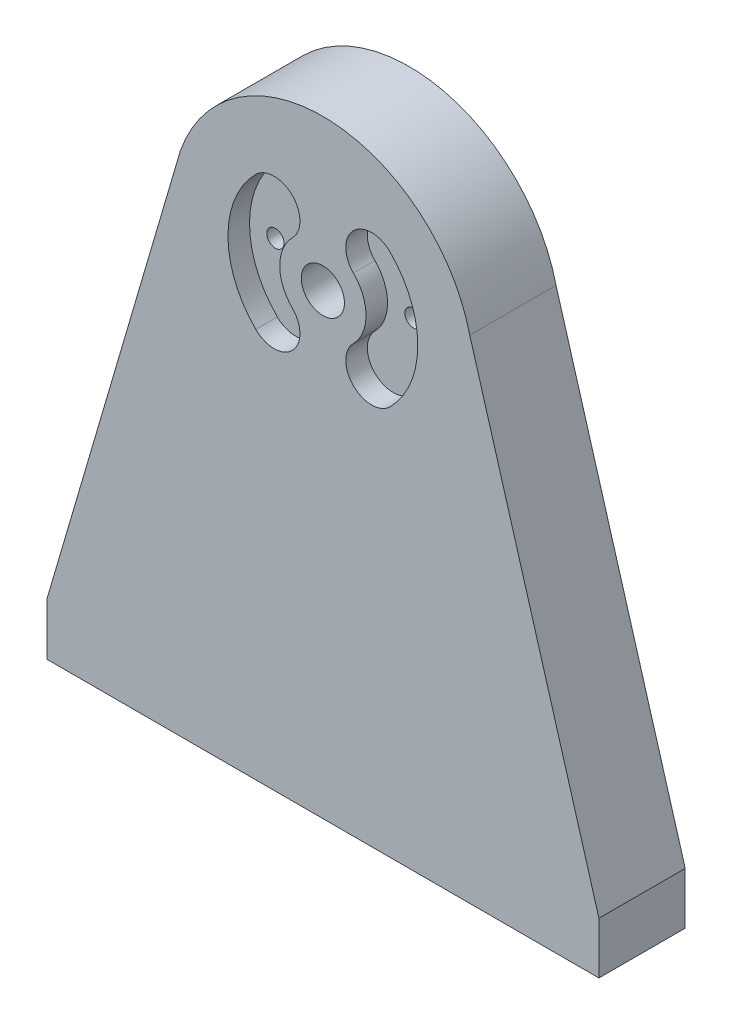
ISO-10303-21;
HEADER;
FILE_DESCRIPTION(('STEP AP214'),'2;1');
FILE_NAME('part.step','',(''),(''),'','','');
FILE_SCHEMA(('AUTOMOTIVE_DESIGN { 1 0 10303 214 1 1 1 1 }'));
ENDSEC;
DATA;
#1=APPLICATION_CONTEXT('core data for automotive mechanical design processes');
#2=APPLICATION_PROTOCOL_DEFINITION('international standard','automotive_design',2000,#1);
#3=PRODUCT_CONTEXT('',#1,'mechanical');
#4=PRODUCT('Part','Part','',(#3));
#5=PRODUCT_RELATED_PRODUCT_CATEGORY('part','',(#4));
#6=PRODUCT_DEFINITION_FORMATION('','',#4);
#7=PRODUCT_DEFINITION_CONTEXT('part definition',#1,'design');
#8=PRODUCT_DEFINITION('design','',#6,#7);
#9=PRODUCT_DEFINITION_SHAPE('','',#8);
#10=(LENGTH_UNIT() NAMED_UNIT(*) SI_UNIT(.MILLI.,.METRE.));
#11=(NAMED_UNIT(*) PLANE_ANGLE_UNIT() SI_UNIT($,.RADIAN.));
#12=(NAMED_UNIT(*) SI_UNIT($,.STERADIAN.) SOLID_ANGLE_UNIT());
#13=UNCERTAINTY_MEASURE_WITH_UNIT(LENGTH_MEASURE(1.E-05),#10,'distance_accuracy_value','');
#14=(GEOMETRIC_REPRESENTATION_CONTEXT(3) GLOBAL_UNCERTAINTY_ASSIGNED_CONTEXT((#13)) GLOBAL_UNIT_ASSIGNED_CONTEXT((#10,
#11,#12)) REPRESENTATION_CONTEXT('',''));
#15=CARTESIAN_POINT('',(0.,0.,0.));
#16=DIRECTION('',(0.,0.,1.));
#17=DIRECTION('',(1.,0.,0.));
#18=AXIS2_PLACEMENT_3D('',#15,#16,#17);
#19=CARTESIAN_POINT('',(8.,55.,5.));
#20=DIRECTION('',(0.,-1.,0.));
#21=DIRECTION('',(0.,0.,-1.));
#22=AXIS2_PLACEMENT_3D('',#19,#20,#21);
#23=CYLINDRICAL_SURFACE('',#22,1.);
#24=CARTESIAN_POINT('',(8.,0.,5.));
#25=DIRECTION('',(0.,-1.,0.));
#26=DIRECTION('',(0.,0.,-1.));
#27=AXIS2_PLACEMENT_3D('',#24,#25,#26);
#28=CIRCLE('',#27,1.);
#29=CARTESIAN_POINT('',(8.,0.,4.));
#30=VERTEX_POINT('',#29);
#31=EDGE_CURVE('E264',#30,#30,#28,.T.);
#32=ORIENTED_EDGE('',*,*,#31,.T.);
#33=EDGE_LOOP('',(#32));
#34=FACE_BOUND('',#33,.T.);
#35=CARTESIAN_POINT('',(8.,53.,5.));
#36=DIRECTION('',(0.,-0.707106781186547,-0.707106781186547));
#37=DIRECTION('',(0.,-0.707106781186547,0.707106781186547));
#38=AXIS2_PLACEMENT_3D('',#35,#36,#37);
#39=ELLIPSE('',#38,1.4142135623731,1.);
#40=CARTESIAN_POINT('',(7.,53.,5.));
#41=VERTEX_POINT('',#40);
#42=CARTESIAN_POINT('',(9.,53.,5.));
#43=VERTEX_POINT('',#42);
#44=EDGE_CURVE('E62',#41,#43,#39,.F.);
#45=ORIENTED_EDGE('',*,*,#44,.T.);
#46=CARTESIAN_POINT('',(8.,53.,5.));
#47=DIRECTION('',(0.,-0.707106781186547,0.707106781186547));
#48=DIRECTION('',(0.,-0.707106781186547,-0.707106781186547));
#49=AXIS2_PLACEMENT_3D('',#46,#47,#48);
#50=ELLIPSE('',#49,1.4142135623731,1.);
#51=EDGE_CURVE('E187',#43,#41,#50,.F.);
#52=ORIENTED_EDGE('',*,*,#51,.T.);
#53=EDGE_LOOP('',(#45,#52));
#54=FACE_BOUND('',#53,.T.);
#55=ADVANCED_FACE('F44',(#34,#54),#23,.F.);
#56=CARTESIAN_POINT('',(-8.,55.,5.));
#57=DIRECTION('',(0.,-1.,0.));
#58=DIRECTION('',(0.,0.,-1.));
#59=AXIS2_PLACEMENT_3D('',#56,#57,#58);
#60=CYLINDRICAL_SURFACE('',#59,1.);
#61=CARTESIAN_POINT('',(-8.,0.,5.));
#62=DIRECTION('',(0.,-1.,0.));
#63=DIRECTION('',(0.,0.,-1.));
#64=AXIS2_PLACEMENT_3D('',#61,#62,#63);
#65=CIRCLE('',#64,1.);
#66=CARTESIAN_POINT('',(-8.,0.,4.));
#67=VERTEX_POINT('',#66);
#68=EDGE_CURVE('E259',#67,#67,#65,.T.);
#69=ORIENTED_EDGE('',*,*,#68,.T.);
#70=EDGE_LOOP('',(#69));
#71=FACE_BOUND('',#70,.T.);
#72=CARTESIAN_POINT('',(-8.,53.,5.));
#73=DIRECTION('',(0.,-0.707106781186547,-0.707106781186547));
#74=DIRECTION('',(0.,-0.707106781186547,0.707106781186547));
#75=AXIS2_PLACEMENT_3D('',#72,#73,#74);
#76=ELLIPSE('',#75,1.41421356237309,1.);
#77=CARTESIAN_POINT('',(-9.,53.,5.));
#78=VERTEX_POINT('',#77);
#79=CARTESIAN_POINT('',(-7.,53.,5.));
#80=VERTEX_POINT('',#79);
#81=EDGE_CURVE('E69',#78,#80,#76,.F.);
#82=ORIENTED_EDGE('',*,*,#81,.T.);
#83=CARTESIAN_POINT('',(-8.,53.,5.));
#84=DIRECTION('',(0.,-0.707106781186547,0.707106781186547));
#85=DIRECTION('',(0.,-0.707106781186547,-0.707106781186547));
#86=AXIS2_PLACEMENT_3D('',#83,#84,#85);
#87=ELLIPSE('',#86,1.41421356237309,1.);
#88=EDGE_CURVE('E163',#80,#78,#87,.F.);
#89=ORIENTED_EDGE('',*,*,#88,.T.);
#90=EDGE_LOOP('',(#82,#89));
#91=FACE_BOUND('',#90,.T.);
#92=ADVANCED_FACE('F173',(#71,#91),#60,.F.);
#93=CARTESIAN_POINT('',(0.,53.,10.));
#94=DIRECTION('',(0.,0.,1.));
#95=DIRECTION('',(1.,0.,0.));
#96=AXIS2_PLACEMENT_3D('',#93,#94,#95);
#97=PLANE('',#96);
#98=CARTESIAN_POINT('',(5.65685424949238,58.6568542494924,10.));
#99=DIRECTION('',(0.,0.,1.));
#100=DIRECTION('',(-1.,0.,0.));
#101=AXIS2_PLACEMENT_3D('',#98,#99,#100);
#102=CIRCLE('',#101,3.);
#103=CARTESIAN_POINT('',(7.77817459305203,60.778174593052,10.));
#104=VERTEX_POINT('',#103);
#105=CARTESIAN_POINT('',(3.53553390593274,56.5355339059327,10.));
#106=VERTEX_POINT('',#105);
#107=EDGE_CURVE('E188',#104,#106,#102,.T.);
#108=ORIENTED_EDGE('',*,*,#107,.F.);
#109=CARTESIAN_POINT('',(0.,53.,10.));
#110=DIRECTION('',(0.,0.,1.));
#111=DIRECTION('',(1.,0.,0.));
#112=AXIS2_PLACEMENT_3D('',#109,#110,#111);
#113=CIRCLE('',#112,11.);
#114=CARTESIAN_POINT('',(7.77817459305202,45.221825406948,10.));
#115=VERTEX_POINT('',#114);
#116=EDGE_CURVE('E230',#115,#104,#113,.T.);
#117=ORIENTED_EDGE('',*,*,#116,.F.);
#118=CARTESIAN_POINT('',(5.65685424949238,47.3431457505076,10.));
#119=DIRECTION('',(0.,0.,1.));
#120=DIRECTION('',(1.,0.,0.));
#121=AXIS2_PLACEMENT_3D('',#118,#119,#120);
#122=CIRCLE('',#121,3.);
#123=CARTESIAN_POINT('',(3.53553390593273,49.4644660940673,10.));
#124=VERTEX_POINT('',#123);
#125=EDGE_CURVE('E242',#124,#115,#122,.T.);
#126=ORIENTED_EDGE('',*,*,#125,.F.);
#127=CARTESIAN_POINT('',(0.,53.,10.));
#128=DIRECTION('',(0.,0.,-1.));
#129=DIRECTION('',(1.,0.,0.));
#130=AXIS2_PLACEMENT_3D('',#127,#128,#129);
#131=CIRCLE('',#130,5.);
#132=EDGE_CURVE('E236',#106,#124,#131,.T.);
#133=ORIENTED_EDGE('',*,*,#132,.F.);
#134=EDGE_LOOP('',(#108,#117,#126,#133));
#135=FACE_BOUND('',#134,.T.);
#136=CARTESIAN_POINT('',(0.,53.,10.));
#137=DIRECTION('',(0.,0.,1.));
#138=DIRECTION('',(1.,0.,0.));
#139=AXIS2_PLACEMENT_3D('',#136,#137,#138);
#140=CIRCLE('',#139,2.5);
#141=CARTESIAN_POINT('',(2.5,53.,10.));
#142=VERTEX_POINT('',#141);
#143=EDGE_CURVE('E216',#142,#142,#140,.T.);
#144=ORIENTED_EDGE('',*,*,#143,.F.);
#145=EDGE_LOOP('',(#144));
#146=FACE_BOUND('',#145,.T.);
#147=DIRECTION('',(-0.281490106882961,0.959564130075223,0.));
#148=VECTOR('',#147,1.);
#149=CARTESIAN_POINT('',(32.,6.,10.));
#150=LINE('',#149,#148);
#151=CARTESIAN_POINT('',(32.,6.,10.));
#152=VERTEX_POINT('',#151);
#153=CARTESIAN_POINT('',(17.027168618915,57.0404862112172,10.));
#154=VERTEX_POINT('',#153);
#155=EDGE_CURVE('E289',#152,#154,#150,.T.);
#156=ORIENTED_EDGE('',*,*,#155,.T.);
#157=CARTESIAN_POINT('',(0.,53.,10.));
#158=DIRECTION('',(0.,0.,1.));
#159=DIRECTION('',(1.,0.,0.));
#160=AXIS2_PLACEMENT_3D('',#157,#158,#159);
#161=CIRCLE('',#160,17.5);
#162=CARTESIAN_POINT('',(-16.5115497472368,58.7981656534221,10.));
#163=VERTEX_POINT('',#162);
#164=EDGE_CURVE('E292',#154,#163,#161,.T.);
#165=ORIENTED_EDGE('',*,*,#164,.T.);
#166=DIRECTION('',(-0.281490106882961,-0.959564130075223,0.));
#167=VECTOR('',#166,1.);
#168=CARTESIAN_POINT('',(-32.,6.,10.));
#169=LINE('',#168,#167);
#170=CARTESIAN_POINT('',(-32.,6.,10.));
#171=VERTEX_POINT('',#170);
#172=EDGE_CURVE('E294',#163,#171,#169,.T.);
#173=ORIENTED_EDGE('',*,*,#172,.T.);
#174=DIRECTION('',(0.,-1.,0.));
#175=VECTOR('',#174,1.);
#176=CARTESIAN_POINT('',(-32.,0.,10.));
#177=LINE('',#176,#175);
#178=CARTESIAN_POINT('',(-32.,0.,10.));
#179=VERTEX_POINT('',#178);
#180=EDGE_CURVE('E297',#171,#179,#177,.T.);
#181=ORIENTED_EDGE('',*,*,#180,.T.);
#182=DIRECTION('',(1.,0.,0.));
#183=VECTOR('',#182,1.);
#184=CARTESIAN_POINT('',(-32.,0.,10.));
#185=LINE('',#184,#183);
#186=CARTESIAN_POINT('',(32.,0.,10.));
#187=VERTEX_POINT('',#186);
#188=EDGE_CURVE('E298',#179,#187,#185,.T.);
#189=ORIENTED_EDGE('',*,*,#188,.T.);
#190=DIRECTION('',(0.,1.,0.));
#191=VECTOR('',#190,1.);
#192=CARTESIAN_POINT('',(32.,0.,10.));
#193=LINE('',#192,#191);
#194=EDGE_CURVE('E296',#187,#152,#193,.T.);
#195=ORIENTED_EDGE('',*,*,#194,.T.);
#196=EDGE_LOOP('',(#156,#165,#173,#181,#189,#195));
#197=FACE_BOUND('',#196,.T.);
#198=CARTESIAN_POINT('',(-5.65685424949238,47.3431457505076,10.));
#199=DIRECTION('',(0.,0.,1.));
#200=DIRECTION('',(-1.,0.,0.));
#201=AXIS2_PLACEMENT_3D('',#198,#199,#200);
#202=CIRCLE('',#201,3.);
#203=CARTESIAN_POINT('',(-7.77817459305202,45.221825406948,10.));
#204=VERTEX_POINT('',#203);
#205=CARTESIAN_POINT('',(-3.53553390593274,49.4644660940673,10.));
#206=VERTEX_POINT('',#205);
#207=EDGE_CURVE('E201',#204,#206,#202,.T.);
#208=ORIENTED_EDGE('',*,*,#207,.F.);
#209=CARTESIAN_POINT('',(0.,53.,10.));
#210=DIRECTION('',(0.,0.,1.));
#211=DIRECTION('',(1.,0.,0.));
#212=AXIS2_PLACEMENT_3D('',#209,#210,#211);
#213=CIRCLE('',#212,11.);
#214=CARTESIAN_POINT('',(-7.77817459305202,60.778174593052,10.));
#215=VERTEX_POINT('',#214);
#216=EDGE_CURVE('E194',#215,#204,#213,.T.);
#217=ORIENTED_EDGE('',*,*,#216,.F.);
#218=CARTESIAN_POINT('',(-5.65685424949238,58.6568542494924,10.));
#219=DIRECTION('',(0.,0.,1.));
#220=DIRECTION('',(1.,0.,0.));
#221=AXIS2_PLACEMENT_3D('',#218,#219,#220);
#222=CIRCLE('',#221,3.);
#223=CARTESIAN_POINT('',(-3.53553390593274,56.5355339059327,10.));
#224=VERTEX_POINT('',#223);
#225=EDGE_CURVE('E207',#224,#215,#222,.T.);
#226=ORIENTED_EDGE('',*,*,#225,.F.);
#227=CARTESIAN_POINT('',(0.,53.,10.));
#228=DIRECTION('',(0.,0.,-1.));
#229=DIRECTION('',(1.,0.,0.));
#230=AXIS2_PLACEMENT_3D('',#227,#228,#229);
#231=CIRCLE('',#230,5.00000000000001);
#232=EDGE_CURVE('E202',#206,#224,#231,.T.);
#233=ORIENTED_EDGE('',*,*,#232,.F.);
#234=EDGE_LOOP('',(#208,#217,#226,#233));
#235=FACE_BOUND('',#234,.T.);
#236=ADVANCED_FACE('F371',(#135,#146,#197,#235),#97,.T.);
#237=CARTESIAN_POINT('',(32.,6.,10.));
#238=DIRECTION('',(-0.959564130075223,-0.281490106882961,0.));
#239=DIRECTION('',(0.281490106882961,-0.959564130075223,0.));
#240=AXIS2_PLACEMENT_3D('',#237,#238,#239);
#241=PLANE('',#240);
#242=DIRECTION('',(-0.281490106882961,0.959564130075223,0.));
#243=VECTOR('',#242,1.);
#244=CARTESIAN_POINT('',(32.,6.,0.));
#245=LINE('',#244,#243);
#246=CARTESIAN_POINT('',(32.,6.,0.));
#247=VERTEX_POINT('',#246);
#248=CARTESIAN_POINT('',(17.027168618915,57.0404862112172,0.));
#249=VERTEX_POINT('',#248);
#250=EDGE_CURVE('E280',#247,#249,#245,.T.);
#251=ORIENTED_EDGE('',*,*,#250,.T.);
#252=DIRECTION('',(0.,0.,-1.));
#253=VECTOR('',#252,1.);
#254=CARTESIAN_POINT('',(17.027168618915,57.0404862112172,10.));
#255=LINE('',#254,#253);
#256=EDGE_CURVE('E11',#154,#249,#255,.T.);
#257=ORIENTED_EDGE('',*,*,#256,.F.);
#258=ORIENTED_EDGE('',*,*,#155,.F.);
#259=DIRECTION('',(0.,0.,-1.));
#260=VECTOR('',#259,1.);
#261=CARTESIAN_POINT('',(32.,6.,10.));
#262=LINE('',#261,#260);
#263=EDGE_CURVE('E305',#152,#247,#262,.T.);
#264=ORIENTED_EDGE('',*,*,#263,.T.);
#265=EDGE_LOOP('',(#251,#257,#258,#264));
#266=FACE_BOUND('',#265,.T.);
#267=ADVANCED_FACE('F50',(#266),#241,.F.);
#268=CARTESIAN_POINT('',(0.,53.,10.));
#269=DIRECTION('',(0.,0.,-1.));
#270=DIRECTION('',(-1.,0.,0.));
#271=AXIS2_PLACEMENT_3D('',#268,#269,#270);
#272=CYLINDRICAL_SURFACE('',#271,17.5);
#273=CARTESIAN_POINT('',(0.,53.,0.));
#274=DIRECTION('',(0.,0.,1.));
#275=DIRECTION('',(1.,0.,0.));
#276=AXIS2_PLACEMENT_3D('',#273,#274,#275);
#277=CIRCLE('',#276,17.5);
#278=CARTESIAN_POINT('',(-16.5115497472368,58.7981656534221,0.));
#279=VERTEX_POINT('',#278);
#280=EDGE_CURVE('E303',#249,#279,#277,.T.);
#281=ORIENTED_EDGE('',*,*,#280,.T.);
#282=DIRECTION('',(0.,0.,-1.));
#283=VECTOR('',#282,1.);
#284=CARTESIAN_POINT('',(-16.5115497472368,58.7981656534221,10.));
#285=LINE('',#284,#283);
#286=EDGE_CURVE('E53',#163,#279,#285,.T.);
#287=ORIENTED_EDGE('',*,*,#286,.F.);
#288=ORIENTED_EDGE('',*,*,#164,.F.);
#289=ORIENTED_EDGE('',*,*,#256,.T.);
#290=EDGE_LOOP('',(#281,#287,#288,#289));
#291=FACE_BOUND('',#290,.T.);
#292=ADVANCED_FACE('F381',(#291),#272,.T.);
#293=CARTESIAN_POINT('',(-32.,6.,10.));
#294=DIRECTION('',(0.959564130075223,-0.281490106882961,0.));
#295=DIRECTION('',(0.281490106882961,0.959564130075223,0.));
#296=AXIS2_PLACEMENT_3D('',#293,#294,#295);
#297=PLANE('',#296);
#298=DIRECTION('',(-0.281490106882961,-0.959564130075223,0.));
#299=VECTOR('',#298,1.);
#300=CARTESIAN_POINT('',(-32.,6.,0.));
#301=LINE('',#300,#299);
#302=CARTESIAN_POINT('',(-32.,6.,0.));
#303=VERTEX_POINT('',#302);
#304=EDGE_CURVE('E307',#279,#303,#301,.T.);
#305=ORIENTED_EDGE('',*,*,#304,.T.);
#306=DIRECTION('',(0.,0.,-1.));
#307=VECTOR('',#306,1.);
#308=CARTESIAN_POINT('',(-32.,6.,10.));
#309=LINE('',#308,#307);
#310=EDGE_CURVE('E325',#171,#303,#309,.T.);
#311=ORIENTED_EDGE('',*,*,#310,.F.);
#312=ORIENTED_EDGE('',*,*,#172,.F.);
#313=ORIENTED_EDGE('',*,*,#286,.T.);
#314=EDGE_LOOP('',(#305,#311,#312,#313));
#315=FACE_BOUND('',#314,.T.);
#316=ADVANCED_FACE('F377',(#315),#297,.F.);
#317=CARTESIAN_POINT('',(-32.,0.,10.));
#318=DIRECTION('',(1.,0.,0.));
#319=DIRECTION('',(0.,0.,-1.));
#320=AXIS2_PLACEMENT_3D('',#317,#318,#319);
#321=PLANE('',#320);
#322=DIRECTION('',(0.,-1.,0.));
#323=VECTOR('',#322,1.);
#324=CARTESIAN_POINT('',(-32.,0.,0.));
#325=LINE('',#324,#323);
#326=CARTESIAN_POINT('',(-32.,0.,0.));
#327=VERTEX_POINT('',#326);
#328=EDGE_CURVE('E310',#303,#327,#325,.T.);
#329=ORIENTED_EDGE('',*,*,#328,.T.);
#330=DIRECTION('',(0.,0.,-1.));
#331=VECTOR('',#330,1.);
#332=CARTESIAN_POINT('',(-32.,0.,10.));
#333=LINE('',#332,#331);
#334=EDGE_CURVE('E317',#179,#327,#333,.T.);
#335=ORIENTED_EDGE('',*,*,#334,.F.);
#336=ORIENTED_EDGE('',*,*,#180,.F.);
#337=ORIENTED_EDGE('',*,*,#310,.T.);
#338=EDGE_LOOP('',(#329,#335,#336,#337));
#339=FACE_BOUND('',#338,.T.);
#340=ADVANCED_FACE('F355',(#339),#321,.F.);
#341=CARTESIAN_POINT('',(-32.,0.,10.));
#342=DIRECTION('',(0.,1.,0.));
#343=DIRECTION('',(0.,0.,1.));
#344=AXIS2_PLACEMENT_3D('',#341,#342,#343);
#345=PLANE('',#344);
#346=ORIENTED_EDGE('',*,*,#68,.F.);
#347=EDGE_LOOP('',(#346));
#348=FACE_BOUND('',#347,.T.);
#349=ORIENTED_EDGE('',*,*,#31,.F.);
#350=EDGE_LOOP('',(#349));
#351=FACE_BOUND('',#350,.T.);
#352=CARTESIAN_POINT('',(22.,0.,5.));
#353=DIRECTION('',(0.,-1.,0.));
#354=DIRECTION('',(0.,0.,-1.));
#355=AXIS2_PLACEMENT_3D('',#352,#353,#354);
#356=CIRCLE('',#355,2.5);
#357=CARTESIAN_POINT('',(22.,0.,2.5));
#358=VERTEX_POINT('',#357);
#359=EDGE_CURVE('E279',#358,#358,#356,.T.);
#360=ORIENTED_EDGE('',*,*,#359,.F.);
#361=EDGE_LOOP('',(#360));
#362=FACE_BOUND('',#361,.T.);
#363=CARTESIAN_POINT('',(-22.,0.,5.));
#364=DIRECTION('',(0.,-1.,0.));
#365=DIRECTION('',(0.,0.,-1.));
#366=AXIS2_PLACEMENT_3D('',#363,#364,#365);
#367=CIRCLE('',#366,2.5);
#368=CARTESIAN_POINT('',(-22.,0.,2.5));
#369=VERTEX_POINT('',#368);
#370=EDGE_CURVE('E284',#369,#369,#367,.T.);
#371=ORIENTED_EDGE('',*,*,#370,.F.);
#372=EDGE_LOOP('',(#371));
#373=FACE_BOUND('',#372,.T.);
#374=DIRECTION('',(1.,0.,0.));
#375=VECTOR('',#374,1.);
#376=CARTESIAN_POINT('',(-32.,0.,0.));
#377=LINE('',#376,#375);
#378=CARTESIAN_POINT('',(32.,0.,0.));
#379=VERTEX_POINT('',#378);
#380=EDGE_CURVE('E313',#327,#379,#377,.T.);
#381=ORIENTED_EDGE('',*,*,#380,.T.);
#382=DIRECTION('',(0.,0.,-1.));
#383=VECTOR('',#382,1.);
#384=CARTESIAN_POINT('',(32.,0.,10.));
#385=LINE('',#384,#383);
#386=EDGE_CURVE('E316',#187,#379,#385,.T.);
#387=ORIENTED_EDGE('',*,*,#386,.F.);
#388=ORIENTED_EDGE('',*,*,#188,.F.);
#389=ORIENTED_EDGE('',*,*,#334,.T.);
#390=EDGE_LOOP('',(#381,#387,#388,#389));
#391=FACE_BOUND('',#390,.T.);
#392=ADVANCED_FACE('F346',(#348,#351,#362,#373,#391),#345,.F.);
#393=CARTESIAN_POINT('',(32.,0.,10.));
#394=DIRECTION('',(-1.,0.,0.));
#395=DIRECTION('',(0.,0.,1.));
#396=AXIS2_PLACEMENT_3D('',#393,#394,#395);
#397=PLANE('',#396);
#398=DIRECTION('',(0.,1.,0.));
#399=VECTOR('',#398,1.);
#400=CARTESIAN_POINT('',(32.,0.,0.));
#401=LINE('',#400,#399);
#402=EDGE_CURVE('E295',#379,#247,#401,.T.);
#403=ORIENTED_EDGE('',*,*,#402,.T.);
#404=ORIENTED_EDGE('',*,*,#263,.F.);
#405=ORIENTED_EDGE('',*,*,#194,.F.);
#406=ORIENTED_EDGE('',*,*,#386,.T.);
#407=EDGE_LOOP('',(#403,#404,#405,#406));
#408=FACE_BOUND('',#407,.T.);
#409=ADVANCED_FACE('F352',(#408),#397,.F.);
#410=CARTESIAN_POINT('',(0.,53.,0.));
#411=DIRECTION('',(0.,0.,1.));
#412=DIRECTION('',(1.,0.,0.));
#413=AXIS2_PLACEMENT_3D('',#410,#411,#412);
#414=PLANE('',#413);
#415=CARTESIAN_POINT('',(0.,53.,0.));
#416=DIRECTION('',(0.,0.,1.));
#417=DIRECTION('',(1.,0.,0.));
#418=AXIS2_PLACEMENT_3D('',#415,#416,#417);
#419=CIRCLE('',#418,2.5);
#420=CARTESIAN_POINT('',(2.5,53.,0.));
#421=VERTEX_POINT('',#420);
#422=EDGE_CURVE('E47',#421,#421,#419,.T.);
#423=ORIENTED_EDGE('',*,*,#422,.T.);
#424=EDGE_LOOP('',(#423));
#425=FACE_BOUND('',#424,.T.);
#426=ORIENTED_EDGE('',*,*,#250,.F.);
#427=ORIENTED_EDGE('',*,*,#402,.F.);
#428=ORIENTED_EDGE('',*,*,#380,.F.);
#429=ORIENTED_EDGE('',*,*,#328,.F.);
#430=ORIENTED_EDGE('',*,*,#304,.F.);
#431=ORIENTED_EDGE('',*,*,#280,.F.);
#432=EDGE_LOOP('',(#426,#427,#428,#429,#430,#431));
#433=FACE_BOUND('',#432,.T.);
#434=ADVANCED_FACE('F341',(#425,#433),#414,.F.);
#435=CARTESIAN_POINT('',(-22.,10.,5.));
#436=DIRECTION('',(0.,-1.,0.));
#437=DIRECTION('',(0.,0.,-1.));
#438=AXIS2_PLACEMENT_3D('',#435,#436,#437);
#439=CYLINDRICAL_SURFACE('',#438,2.5);
#440=CARTESIAN_POINT('',(-22.,10.,5.));
#441=DIRECTION('',(0.,-1.,0.));
#442=DIRECTION('',(0.,0.,-1.));
#443=AXIS2_PLACEMENT_3D('',#440,#441,#442);
#444=CIRCLE('',#443,2.5);
#445=CARTESIAN_POINT('',(-22.,10.,2.5));
#446=VERTEX_POINT('',#445);
#447=EDGE_CURVE('E282',#446,#446,#444,.T.);
#448=ORIENTED_EDGE('',*,*,#447,.F.);
#449=EDGE_LOOP('',(#448));
#450=FACE_BOUND('',#449,.T.);
#451=ORIENTED_EDGE('',*,*,#370,.T.);
#452=EDGE_LOOP('',(#451));
#453=FACE_BOUND('',#452,.T.);
#454=ADVANCED_FACE('F338',(#450,#453),#439,.F.);
#455=CARTESIAN_POINT('',(-22.,10.,5.));
#456=DIRECTION('',(0.,-1.,0.));
#457=DIRECTION('',(0.,0.,-1.));
#458=AXIS2_PLACEMENT_3D('',#455,#456,#457);
#459=PLANE('',#458);
#460=CARTESIAN_POINT('',(-22.,10.,5.));
#461=DIRECTION('',(0.,-1.,0.));
#462=DIRECTION('',(0.,0.,-1.));
#463=AXIS2_PLACEMENT_3D('',#460,#461,#462);
#464=CIRCLE('',#463,2.1);
#465=CARTESIAN_POINT('',(-22.,10.,2.9));
#466=VERTEX_POINT('',#465);
#467=EDGE_CURVE('E290',#466,#466,#464,.T.);
#468=ORIENTED_EDGE('',*,*,#467,.F.);
#469=EDGE_LOOP('',(#468));
#470=FACE_BOUND('',#469,.T.);
#471=ORIENTED_EDGE('',*,*,#447,.T.);
#472=EDGE_LOOP('',(#471));
#473=FACE_BOUND('',#472,.T.);
#474=ADVANCED_FACE('F331',(#470,#473),#459,.T.);
#475=CARTESIAN_POINT('',(22.,10.,5.));
#476=DIRECTION('',(0.,-1.,0.));
#477=DIRECTION('',(0.,0.,-1.));
#478=AXIS2_PLACEMENT_3D('',#475,#476,#477);
#479=CYLINDRICAL_SURFACE('',#478,2.5);
#480=CARTESIAN_POINT('',(22.,10.,5.));
#481=DIRECTION('',(0.,-1.,0.));
#482=DIRECTION('',(0.,0.,-1.));
#483=AXIS2_PLACEMENT_3D('',#480,#481,#482);
#484=CIRCLE('',#483,2.5);
#485=CARTESIAN_POINT('',(22.,10.,2.5));
#486=VERTEX_POINT('',#485);
#487=EDGE_CURVE('E273',#486,#486,#484,.T.);
#488=ORIENTED_EDGE('',*,*,#487,.F.);
#489=EDGE_LOOP('',(#488));
#490=FACE_BOUND('',#489,.T.);
#491=ORIENTED_EDGE('',*,*,#359,.T.);
#492=EDGE_LOOP('',(#491));
#493=FACE_BOUND('',#492,.T.);
#494=ADVANCED_FACE('F340',(#490,#493),#479,.F.);
#495=CARTESIAN_POINT('',(22.,10.,5.));
#496=DIRECTION('',(0.,-1.,0.));
#497=DIRECTION('',(0.,0.,-1.));
#498=AXIS2_PLACEMENT_3D('',#495,#496,#497);
#499=PLANE('',#498);
#500=CARTESIAN_POINT('',(22.,10.,5.));
#501=DIRECTION('',(0.,-1.,0.));
#502=DIRECTION('',(0.,0.,-1.));
#503=AXIS2_PLACEMENT_3D('',#500,#501,#502);
#504=CIRCLE('',#503,2.1);
#505=CARTESIAN_POINT('',(22.,10.,2.9));
#506=VERTEX_POINT('',#505);
#507=EDGE_CURVE('E271',#506,#506,#504,.T.);
#508=ORIENTED_EDGE('',*,*,#507,.F.);
#509=EDGE_LOOP('',(#508));
#510=FACE_BOUND('',#509,.T.);
#511=ORIENTED_EDGE('',*,*,#487,.T.);
#512=EDGE_LOOP('',(#511));
#513=FACE_BOUND('',#512,.T.);
#514=ADVANCED_FACE('F581',(#510,#513),#499,.T.);
#515=CARTESIAN_POINT('',(22.,12.4,5.));
#516=DIRECTION('',(0.,-1.,0.));
#517=DIRECTION('',(0.,0.,-1.));
#518=AXIS2_PLACEMENT_3D('',#515,#516,#517);
#519=CYLINDRICAL_SURFACE('',#518,2.1);
#520=CARTESIAN_POINT('',(22.,12.4,5.));
#521=DIRECTION('',(0.,-1.,0.));
#522=DIRECTION('',(0.,0.,-1.));
#523=AXIS2_PLACEMENT_3D('',#520,#521,#522);
#524=CIRCLE('',#523,2.1);
#525=CARTESIAN_POINT('',(22.,12.4,2.9));
#526=VERTEX_POINT('',#525);
#527=EDGE_CURVE('E268',#526,#526,#524,.T.);
#528=CARTESIAN_POINT('',(22.,10.,2.9));
#529=CARTESIAN_POINT('',(22.,10.025,2.9));
#530=CARTESIAN_POINT('',(22.,10.05,2.9));
#531=CARTESIAN_POINT('',(22.,10.1,2.9));
#532=CARTESIAN_POINT('',(22.,10.125,2.9));
#533=CARTESIAN_POINT('',(22.,10.175,2.9));
#534=CARTESIAN_POINT('',(22.,10.2,2.9));
#535=CARTESIAN_POINT('',(22.,10.25,2.9));
#536=CARTESIAN_POINT('',(22.,10.275,2.9));
#537=CARTESIAN_POINT('',(22.,10.325,2.9));
#538=CARTESIAN_POINT('',(22.,10.35,2.9));
#539=CARTESIAN_POINT('',(22.,10.4,2.9));
#540=CARTESIAN_POINT('',(22.,10.425,2.9));
#541=CARTESIAN_POINT('',(22.,10.475,2.9));
#542=CARTESIAN_POINT('',(22.,10.5,2.9));
#543=CARTESIAN_POINT('',(22.,10.55,2.9));
#544=CARTESIAN_POINT('',(22.,10.575,2.9));
#545=CARTESIAN_POINT('',(22.,10.625,2.9));
#546=CARTESIAN_POINT('',(22.,10.65,2.9));
#547=CARTESIAN_POINT('',(22.,10.7,2.9));
#548=CARTESIAN_POINT('',(22.,10.725,2.9));
#549=CARTESIAN_POINT('',(22.,10.775,2.9));
#550=CARTESIAN_POINT('',(22.,10.8,2.9));
#551=CARTESIAN_POINT('',(22.,10.85,2.9));
#552=CARTESIAN_POINT('',(22.,10.875,2.9));
#553=CARTESIAN_POINT('',(22.,10.925,2.9));
#554=CARTESIAN_POINT('',(22.,10.95,2.9));
#555=CARTESIAN_POINT('',(22.,11.,2.9));
#556=CARTESIAN_POINT('',(22.,11.025,2.9));
#557=CARTESIAN_POINT('',(22.,11.075,2.9));
#558=CARTESIAN_POINT('',(22.,11.1,2.9));
#559=CARTESIAN_POINT('',(22.,11.15,2.9));
#560=CARTESIAN_POINT('',(22.,11.175,2.9));
#561=CARTESIAN_POINT('',(22.,11.225,2.9));
#562=CARTESIAN_POINT('',(22.,11.25,2.9));
#563=CARTESIAN_POINT('',(22.,11.3,2.9));
#564=CARTESIAN_POINT('',(22.,11.325,2.9));
#565=CARTESIAN_POINT('',(22.,11.375,2.9));
#566=CARTESIAN_POINT('',(22.,11.4,2.9));
#567=CARTESIAN_POINT('',(22.,11.45,2.9));
#568=CARTESIAN_POINT('',(22.,11.475,2.9));
#569=CARTESIAN_POINT('',(22.,11.525,2.9));
#570=CARTESIAN_POINT('',(22.,11.55,2.9));
#571=CARTESIAN_POINT('',(22.,11.6,2.9));
#572=CARTESIAN_POINT('',(22.,11.625,2.9));
#573=CARTESIAN_POINT('',(22.,11.675,2.9));
#574=CARTESIAN_POINT('',(22.,11.7,2.9));
#575=CARTESIAN_POINT('',(22.,11.75,2.9));
#576=CARTESIAN_POINT('',(22.,11.775,2.9));
#577=CARTESIAN_POINT('',(22.,11.825,2.9));
#578=CARTESIAN_POINT('',(22.,11.85,2.9));
#579=CARTESIAN_POINT('',(22.,11.9,2.9));
#580=CARTESIAN_POINT('',(22.,11.925,2.9));
#581=CARTESIAN_POINT('',(22.,11.975,2.9));
#582=CARTESIAN_POINT('',(22.,12.,2.9));
#583=CARTESIAN_POINT('',(22.,12.05,2.9));
#584=CARTESIAN_POINT('',(22.,12.075,2.9));
#585=CARTESIAN_POINT('',(22.,12.125,2.9));
#586=CARTESIAN_POINT('',(22.,12.15,2.9));
#587=CARTESIAN_POINT('',(22.,12.2,2.9));
#588=CARTESIAN_POINT('',(22.,12.225,2.9));
#589=CARTESIAN_POINT('',(22.,12.275,2.9));
#590=CARTESIAN_POINT('',(22.,12.3,2.9));
#591=CARTESIAN_POINT('',(22.,12.35,2.9));
#592=CARTESIAN_POINT('',(22.,12.375,2.9));
#593=CARTESIAN_POINT('',(22.,12.4,2.9));
#594=B_SPLINE_CURVE_WITH_KNOTS('',3,(#528,#529,#530,#531,#532,#533,#534,#535,#536,#537,#538,
#539,#540,#541,#542,#543,#544,#545,#546,#547,#548,#549,#550,#551,#552,#553,#554,#555,#556,#557,
#558,#559,#560,#561,#562,#563,#564,#565,#566,#567,#568,#569,#570,#571,#572,#573,#574,#575,#576,
#577,#578,#579,#580,#581,#582,#583,#584,#585,#586,#587,#588,#589,#590,#591,#592,#593),
.UNSPECIFIED.,.F.,.F.,(4,2,2,2,2,2,2,2,2,2,2,2,2,2,2,2,2,2,2,2,2,2,2,2,2,2,2,2,2,2,2,2,4),(0.,
0.0750000000000004,0.150000000000001,0.225000000000001,0.3,0.375,0.450000000000001,
0.524999999999999,0.6,0.675,0.750000000000001,0.825000000000001,0.9,0.975,1.05,1.125,1.2,1.275,
1.35,1.425,1.5,1.575,1.65,1.725,1.8,1.875,1.95,2.025,2.1,2.175,2.25,2.325,2.4),.UNSPECIFIED.);
#595=EDGE_CURVE('BSEAM605',#506,#526,#594,.T.);
#596=ORIENTED_EDGE('',*,*,#507,.T.);
#597=ORIENTED_EDGE('',*,*,#527,.F.);
#598=ORIENTED_EDGE('',*,*,#595,.T.);
#599=ORIENTED_EDGE('',*,*,#595,.F.);
#600=EDGE_LOOP('',(#596,#598,#597,#599));
#601=FACE_BOUND('',#600,.T.);
#602=ADVANCED_FACE('F605',(#601),#519,.F.);
#603=CARTESIAN_POINT('',(22.,12.4,5.));
#604=DIRECTION('',(0.,-1.,0.));
#605=DIRECTION('',(0.,0.,-1.));
#606=AXIS2_PLACEMENT_3D('',#603,#604,#605);
#607=PLANE('',#606);
#608=ORIENTED_EDGE('',*,*,#527,.T.);
#609=EDGE_LOOP('',(#608));
#610=FACE_BOUND('',#609,.T.);
#611=ADVANCED_FACE('F611',(#610),#607,.T.);
#612=CARTESIAN_POINT('',(-22.,12.4,5.));
#613=DIRECTION('',(0.,-1.,0.));
#614=DIRECTION('',(0.,0.,-1.));
#615=AXIS2_PLACEMENT_3D('',#612,#613,#614);
#616=CYLINDRICAL_SURFACE('',#615,2.1);
#617=CARTESIAN_POINT('',(-22.,12.4,5.));
#618=DIRECTION('',(0.,-1.,0.));
#619=DIRECTION('',(0.,0.,-1.));
#620=AXIS2_PLACEMENT_3D('',#617,#618,#619);
#621=CIRCLE('',#620,2.1);
#622=CARTESIAN_POINT('',(-22.,12.4,2.9));
#623=VERTEX_POINT('',#622);
#624=EDGE_CURVE('E256',#623,#623,#621,.T.);
#625=CARTESIAN_POINT('',(-22.,10.,2.9));
#626=CARTESIAN_POINT('',(-22.,10.025,2.9));
#627=CARTESIAN_POINT('',(-22.,10.05,2.9));
#628=CARTESIAN_POINT('',(-22.,10.1,2.9));
#629=CARTESIAN_POINT('',(-22.,10.125,2.9));
#630=CARTESIAN_POINT('',(-22.,10.175,2.9));
#631=CARTESIAN_POINT('',(-22.,10.2,2.9));
#632=CARTESIAN_POINT('',(-22.,10.25,2.9));
#633=CARTESIAN_POINT('',(-22.,10.275,2.9));
#634=CARTESIAN_POINT('',(-22.,10.325,2.9));
#635=CARTESIAN_POINT('',(-22.,10.35,2.9));
#636=CARTESIAN_POINT('',(-22.,10.4,2.9));
#637=CARTESIAN_POINT('',(-22.,10.425,2.9));
#638=CARTESIAN_POINT('',(-22.,10.475,2.9));
#639=CARTESIAN_POINT('',(-22.,10.5,2.9));
#640=CARTESIAN_POINT('',(-22.,10.55,2.9));
#641=CARTESIAN_POINT('',(-22.,10.575,2.9));
#642=CARTESIAN_POINT('',(-22.,10.625,2.9));
#643=CARTESIAN_POINT('',(-22.,10.65,2.9));
#644=CARTESIAN_POINT('',(-22.,10.7,2.9));
#645=CARTESIAN_POINT('',(-22.,10.725,2.9));
#646=CARTESIAN_POINT('',(-22.,10.775,2.9));
#647=CARTESIAN_POINT('',(-22.,10.8,2.9));
#648=CARTESIAN_POINT('',(-22.,10.85,2.9));
#649=CARTESIAN_POINT('',(-22.,10.875,2.9));
#650=CARTESIAN_POINT('',(-22.,10.925,2.9));
#651=CARTESIAN_POINT('',(-22.,10.95,2.9));
#652=CARTESIAN_POINT('',(-22.,11.,2.9));
#653=CARTESIAN_POINT('',(-22.,11.025,2.9));
#654=CARTESIAN_POINT('',(-22.,11.075,2.9));
#655=CARTESIAN_POINT('',(-22.,11.1,2.9));
#656=CARTESIAN_POINT('',(-22.,11.15,2.9));
#657=CARTESIAN_POINT('',(-22.,11.175,2.9));
#658=CARTESIAN_POINT('',(-22.,11.225,2.9));
#659=CARTESIAN_POINT('',(-22.,11.25,2.9));
#660=CARTESIAN_POINT('',(-22.,11.3,2.9));
#661=CARTESIAN_POINT('',(-22.,11.325,2.9));
#662=CARTESIAN_POINT('',(-22.,11.375,2.9));
#663=CARTESIAN_POINT('',(-22.,11.4,2.9));
#664=CARTESIAN_POINT('',(-22.,11.45,2.9));
#665=CARTESIAN_POINT('',(-22.,11.475,2.9));
#666=CARTESIAN_POINT('',(-22.,11.525,2.9));
#667=CARTESIAN_POINT('',(-22.,11.55,2.9));
#668=CARTESIAN_POINT('',(-22.,11.6,2.9));
#669=CARTESIAN_POINT('',(-22.,11.625,2.9));
#670=CARTESIAN_POINT('',(-22.,11.675,2.9));
#671=CARTESIAN_POINT('',(-22.,11.7,2.9));
#672=CARTESIAN_POINT('',(-22.,11.75,2.9));
#673=CARTESIAN_POINT('',(-22.,11.775,2.9));
#674=CARTESIAN_POINT('',(-22.,11.825,2.9));
#675=CARTESIAN_POINT('',(-22.,11.85,2.9));
#676=CARTESIAN_POINT('',(-22.,11.9,2.9));
#677=CARTESIAN_POINT('',(-22.,11.925,2.9));
#678=CARTESIAN_POINT('',(-22.,11.975,2.9));
#679=CARTESIAN_POINT('',(-22.,12.,2.9));
#680=CARTESIAN_POINT('',(-22.,12.05,2.9));
#681=CARTESIAN_POINT('',(-22.,12.075,2.9));
#682=CARTESIAN_POINT('',(-22.,12.125,2.9));
#683=CARTESIAN_POINT('',(-22.,12.15,2.9));
#684=CARTESIAN_POINT('',(-22.,12.2,2.9));
#685=CARTESIAN_POINT('',(-22.,12.225,2.9));
#686=CARTESIAN_POINT('',(-22.,12.275,2.9));
#687=CARTESIAN_POINT('',(-22.,12.3,2.9));
#688=CARTESIAN_POINT('',(-22.,12.35,2.9));
#689=CARTESIAN_POINT('',(-22.,12.375,2.9));
#690=CARTESIAN_POINT('',(-22.,12.4,2.9));
#691=B_SPLINE_CURVE_WITH_KNOTS('',3,(#625,#626,#627,#628,#629,#630,#631,#632,#633,#634,#635,
#636,#637,#638,#639,#640,#641,#642,#643,#644,#645,#646,#647,#648,#649,#650,#651,#652,#653,#654,
#655,#656,#657,#658,#659,#660,#661,#662,#663,#664,#665,#666,#667,#668,#669,#670,#671,#672,#673,
#674,#675,#676,#677,#678,#679,#680,#681,#682,#683,#684,#685,#686,#687,#688,#689,#690),
.UNSPECIFIED.,.F.,.F.,(4,2,2,2,2,2,2,2,2,2,2,2,2,2,2,2,2,2,2,2,2,2,2,2,2,2,2,2,2,2,2,2,4),(0.,
0.0750000000000004,0.150000000000001,0.225000000000001,0.3,0.375,0.450000000000001,
0.524999999999999,0.6,0.675,0.750000000000001,0.825000000000001,0.9,0.975,1.05,1.125,1.2,1.275,
1.35,1.425,1.5,1.575,1.65,1.725,1.8,1.875,1.95,2.025,2.1,2.175,2.25,2.325,2.4),.UNSPECIFIED.);
#692=EDGE_CURVE('BSEAM332',#466,#623,#691,.T.);
#693=ORIENTED_EDGE('',*,*,#467,.T.);
#694=ORIENTED_EDGE('',*,*,#624,.F.);
#695=ORIENTED_EDGE('',*,*,#692,.T.);
#696=ORIENTED_EDGE('',*,*,#692,.F.);
#697=EDGE_LOOP('',(#693,#695,#694,#696));
#698=FACE_BOUND('',#697,.T.);
#699=ADVANCED_FACE('F332',(#698),#616,.F.);
#700=CARTESIAN_POINT('',(-22.,12.4,5.));
#701=DIRECTION('',(0.,-1.,0.));
#702=DIRECTION('',(0.,0.,-1.));
#703=AXIS2_PLACEMENT_3D('',#700,#701,#702);
#704=PLANE('',#703);
#705=ORIENTED_EDGE('',*,*,#624,.T.);
#706=EDGE_LOOP('',(#705));
#707=FACE_BOUND('',#706,.T.);
#708=ADVANCED_FACE('F479',(#707),#704,.T.);
#709=CARTESIAN_POINT('',(0.,53.,-45.));
#710=DIRECTION('',(0.,0.,1.));
#711=DIRECTION('',(1.,0.,0.));
#712=AXIS2_PLACEMENT_3D('',#709,#710,#711);
#713=CYLINDRICAL_SURFACE('',#712,2.5);
#714=ORIENTED_EDGE('',*,*,#143,.T.);
#715=EDGE_LOOP('',(#714));
#716=FACE_BOUND('',#715,.T.);
#717=ORIENTED_EDGE('',*,*,#422,.F.);
#718=EDGE_LOOP('',(#717));
#719=FACE_BOUND('',#718,.T.);
#720=ADVANCED_FACE('F480',(#716,#719),#713,.F.);
#721=CARTESIAN_POINT('',(5.65685424949238,58.6568542494924,7.5));
#722=DIRECTION('',(0.,0.,1.));
#723=DIRECTION('',(1.,0.,0.));
#724=AXIS2_PLACEMENT_3D('',#721,#722,#723);
#725=CYLINDRICAL_SURFACE('',#724,3.);
#726=ORIENTED_EDGE('',*,*,#107,.T.);
#727=DIRECTION('',(0.,0.,1.));
#728=VECTOR('',#727,1.);
#729=CARTESIAN_POINT('',(3.53553390593274,56.5355339059327,7.5));
#730=LINE('',#729,#728);
#731=CARTESIAN_POINT('',(3.53553390593274,56.5355339059327,7.5));
#732=VERTEX_POINT('',#731);
#733=EDGE_CURVE('E237',#732,#106,#730,.T.);
#734=ORIENTED_EDGE('',*,*,#733,.F.);
#735=CARTESIAN_POINT('',(5.65685424949238,58.6568542494924,7.5));
#736=DIRECTION('',(0.,0.,1.));
#737=DIRECTION('',(-1.,0.,0.));
#738=AXIS2_PLACEMENT_3D('',#735,#736,#737);
#739=CIRCLE('',#738,3.);
#740=CARTESIAN_POINT('',(7.77817459305203,60.778174593052,7.5));
#741=VERTEX_POINT('',#740);
#742=EDGE_CURVE('E224',#741,#732,#739,.T.);
#743=ORIENTED_EDGE('',*,*,#742,.F.);
#744=DIRECTION('',(0.,0.,1.));
#745=VECTOR('',#744,1.);
#746=CARTESIAN_POINT('',(7.77817459305203,60.778174593052,7.5));
#747=LINE('',#746,#745);
#748=EDGE_CURVE('E206',#741,#104,#747,.T.);
#749=ORIENTED_EDGE('',*,*,#748,.T.);
#750=EDGE_LOOP('',(#726,#734,#743,#749));
#751=FACE_BOUND('',#750,.T.);
#752=ADVANCED_FACE('F470',(#751),#725,.F.);
#753=CARTESIAN_POINT('',(0.,53.,7.5));
#754=DIRECTION('',(0.,0.,1.));
#755=DIRECTION('',(1.,0.,0.));
#756=AXIS2_PLACEMENT_3D('',#753,#754,#755);
#757=CYLINDRICAL_SURFACE('',#756,11.);
#758=ORIENTED_EDGE('',*,*,#116,.T.);
#759=ORIENTED_EDGE('',*,*,#748,.F.);
#760=CARTESIAN_POINT('',(0.,53.,7.5));
#761=DIRECTION('',(0.,0.,1.));
#762=DIRECTION('',(1.,0.,0.));
#763=AXIS2_PLACEMENT_3D('',#760,#761,#762);
#764=CIRCLE('',#763,11.);
#765=CARTESIAN_POINT('',(7.77817459305202,45.221825406948,7.5));
#766=VERTEX_POINT('',#765);
#767=EDGE_CURVE('E234',#766,#741,#764,.T.);
#768=ORIENTED_EDGE('',*,*,#767,.F.);
#769=DIRECTION('',(0.,0.,1.));
#770=VECTOR('',#769,1.);
#771=CARTESIAN_POINT('',(7.77817459305202,45.221825406948,7.5));
#772=LINE('',#771,#770);
#773=EDGE_CURVE('E250',#766,#115,#772,.T.);
#774=ORIENTED_EDGE('',*,*,#773,.T.);
#775=EDGE_LOOP('',(#758,#759,#768,#774));
#776=FACE_BOUND('',#775,.T.);
#777=ADVANCED_FACE('F463',(#776),#757,.F.);
#778=CARTESIAN_POINT('',(5.65685424949238,47.3431457505076,7.5));
#779=DIRECTION('',(0.,0.,1.));
#780=DIRECTION('',(1.,0.,0.));
#781=AXIS2_PLACEMENT_3D('',#778,#779,#780);
#782=CYLINDRICAL_SURFACE('',#781,3.);
#783=ORIENTED_EDGE('',*,*,#125,.T.);
#784=ORIENTED_EDGE('',*,*,#773,.F.);
#785=CARTESIAN_POINT('',(5.65685424949238,47.3431457505076,7.5));
#786=DIRECTION('',(0.,0.,1.));
#787=DIRECTION('',(1.,0.,0.));
#788=AXIS2_PLACEMENT_3D('',#785,#786,#787);
#789=CIRCLE('',#788,3.);
#790=CARTESIAN_POINT('',(3.53553390593273,49.4644660940673,7.5));
#791=VERTEX_POINT('',#790);
#792=EDGE_CURVE('E226',#791,#766,#789,.T.);
#793=ORIENTED_EDGE('',*,*,#792,.F.);
#794=DIRECTION('',(0.,0.,1.));
#795=VECTOR('',#794,1.);
#796=CARTESIAN_POINT('',(3.53553390593273,49.4644660940673,7.5));
#797=LINE('',#796,#795);
#798=EDGE_CURVE('E246',#791,#124,#797,.T.);
#799=ORIENTED_EDGE('',*,*,#798,.T.);
#800=EDGE_LOOP('',(#783,#784,#793,#799));
#801=FACE_BOUND('',#800,.T.);
#802=ADVANCED_FACE('F467',(#801),#782,.F.);
#803=CARTESIAN_POINT('',(0.,53.,7.5));
#804=DIRECTION('',(0.,0.,1.));
#805=DIRECTION('',(1.,0.,0.));
#806=AXIS2_PLACEMENT_3D('',#803,#804,#805);
#807=CYLINDRICAL_SURFACE('',#806,5.);
#808=ORIENTED_EDGE('',*,*,#132,.T.);
#809=ORIENTED_EDGE('',*,*,#798,.F.);
#810=CARTESIAN_POINT('',(0.,53.,7.5));
#811=DIRECTION('',(0.,0.,-1.));
#812=DIRECTION('',(1.,0.,0.));
#813=AXIS2_PLACEMENT_3D('',#810,#811,#812);
#814=CIRCLE('',#813,5.);
#815=EDGE_CURVE('E227',#732,#791,#814,.T.);
#816=ORIENTED_EDGE('',*,*,#815,.F.);
#817=ORIENTED_EDGE('',*,*,#733,.T.);
#818=EDGE_LOOP('',(#808,#809,#816,#817));
#819=FACE_BOUND('',#818,.T.);
#820=ADVANCED_FACE('F462',(#819),#807,.T.);
#821=CARTESIAN_POINT('',(2.82842712474619,55.8284271247462,7.5));
#822=DIRECTION('',(0.,0.,-1.));
#823=DIRECTION('',(-1.,0.,0.));
#824=AXIS2_PLACEMENT_3D('',#821,#822,#823);
#825=PLANE('',#824);
#826=CARTESIAN_POINT('',(8.,53.,7.5));
#827=DIRECTION('',(0.,0.,1.));
#828=DIRECTION('',(1.,0.,0.));
#829=AXIS2_PLACEMENT_3D('',#826,#827,#828);
#830=CIRCLE('',#829,1.);
#831=CARTESIAN_POINT('',(9.,53.,7.5));
#832=VERTEX_POINT('',#831);
#833=EDGE_CURVE('E516',#832,#832,#830,.T.);
#834=ORIENTED_EDGE('',*,*,#833,.F.);
#835=EDGE_LOOP('',(#834));
#836=FACE_BOUND('',#835,.T.);
#837=ORIENTED_EDGE('',*,*,#742,.T.);
#838=ORIENTED_EDGE('',*,*,#815,.T.);
#839=ORIENTED_EDGE('',*,*,#792,.T.);
#840=ORIENTED_EDGE('',*,*,#767,.T.);
#841=EDGE_LOOP('',(#837,#838,#839,#840));
#842=FACE_BOUND('',#841,.T.);
#843=ADVANCED_FACE('F460',(#836,#842),#825,.F.);
#844=CARTESIAN_POINT('',(-5.65685424949238,47.3431457505076,7.5));
#845=DIRECTION('',(0.,0.,1.));
#846=DIRECTION('',(1.,0.,0.));
#847=AXIS2_PLACEMENT_3D('',#844,#845,#846);
#848=CYLINDRICAL_SURFACE('',#847,3.);
#849=ORIENTED_EDGE('',*,*,#207,.T.);
#850=DIRECTION('',(0.,0.,1.));
#851=VECTOR('',#850,1.);
#852=CARTESIAN_POINT('',(-3.53553390593274,49.4644660940673,7.5));
#853=LINE('',#852,#851);
#854=CARTESIAN_POINT('',(-3.53553390593274,49.4644660940673,7.5));
#855=VERTEX_POINT('',#854);
#856=EDGE_CURVE('E205',#855,#206,#853,.T.);
#857=ORIENTED_EDGE('',*,*,#856,.F.);
#858=CARTESIAN_POINT('',(-5.65685424949238,47.3431457505076,7.5));
#859=DIRECTION('',(0.,0.,1.));
#860=DIRECTION('',(-1.,0.,0.));
#861=AXIS2_PLACEMENT_3D('',#858,#859,#860);
#862=CIRCLE('',#861,3.);
#863=CARTESIAN_POINT('',(-7.77817459305202,45.221825406948,7.5));
#864=VERTEX_POINT('',#863);
#865=EDGE_CURVE('E189',#864,#855,#862,.T.);
#866=ORIENTED_EDGE('',*,*,#865,.F.);
#867=DIRECTION('',(0.,0.,1.));
#868=VECTOR('',#867,1.);
#869=CARTESIAN_POINT('',(-7.77817459305202,45.221825406948,7.5));
#870=LINE('',#869,#868);
#871=EDGE_CURVE('E212',#864,#204,#870,.T.);
#872=ORIENTED_EDGE('',*,*,#871,.T.);
#873=EDGE_LOOP('',(#849,#857,#866,#872));
#874=FACE_BOUND('',#873,.T.);
#875=ADVANCED_FACE('F450',(#874),#848,.F.);
#876=CARTESIAN_POINT('',(0.,53.,7.5));
#877=DIRECTION('',(0.,0.,1.));
#878=DIRECTION('',(1.,0.,0.));
#879=AXIS2_PLACEMENT_3D('',#876,#877,#878);
#880=CYLINDRICAL_SURFACE('',#879,11.);
#881=ORIENTED_EDGE('',*,*,#216,.T.);
#882=ORIENTED_EDGE('',*,*,#871,.F.);
#883=CARTESIAN_POINT('',(0.,53.,7.5));
#884=DIRECTION('',(0.,0.,1.));
#885=DIRECTION('',(1.,0.,0.));
#886=AXIS2_PLACEMENT_3D('',#883,#884,#885);
#887=CIRCLE('',#886,11.);
#888=CARTESIAN_POINT('',(-7.77817459305202,60.778174593052,7.5));
#889=VERTEX_POINT('',#888);
#890=EDGE_CURVE('E200',#889,#864,#887,.T.);
#891=ORIENTED_EDGE('',*,*,#890,.F.);
#892=DIRECTION('',(0.,0.,1.));
#893=VECTOR('',#892,1.);
#894=CARTESIAN_POINT('',(-7.77817459305202,60.778174593052,7.5));
#895=LINE('',#894,#893);
#896=EDGE_CURVE('E220',#889,#215,#895,.T.);
#897=ORIENTED_EDGE('',*,*,#896,.T.);
#898=EDGE_LOOP('',(#881,#882,#891,#897));
#899=FACE_BOUND('',#898,.T.);
#900=ADVANCED_FACE('F444',(#899),#880,.F.);
#901=CARTESIAN_POINT('',(-5.65685424949238,58.6568542494924,7.5));
#902=DIRECTION('',(0.,0.,1.));
#903=DIRECTION('',(1.,0.,0.));
#904=AXIS2_PLACEMENT_3D('',#901,#902,#903);
#905=CYLINDRICAL_SURFACE('',#904,3.);
#906=ORIENTED_EDGE('',*,*,#225,.T.);
#907=ORIENTED_EDGE('',*,*,#896,.F.);
#908=CARTESIAN_POINT('',(-5.65685424949238,58.6568542494924,7.5));
#909=DIRECTION('',(0.,0.,1.));
#910=DIRECTION('',(1.,0.,0.));
#911=AXIS2_PLACEMENT_3D('',#908,#909,#910);
#912=CIRCLE('',#911,3.);
#913=CARTESIAN_POINT('',(-3.53553390593274,56.5355339059327,7.5));
#914=VERTEX_POINT('',#913);
#915=EDGE_CURVE('E198',#914,#889,#912,.T.);
#916=ORIENTED_EDGE('',*,*,#915,.F.);
#917=DIRECTION('',(0.,0.,1.));
#918=VECTOR('',#917,1.);
#919=CARTESIAN_POINT('',(-3.53553390593274,56.5355339059327,7.5));
#920=LINE('',#919,#918);
#921=EDGE_CURVE('E218',#914,#224,#920,.T.);
#922=ORIENTED_EDGE('',*,*,#921,.T.);
#923=EDGE_LOOP('',(#906,#907,#916,#922));
#924=FACE_BOUND('',#923,.T.);
#925=ADVANCED_FACE('F447',(#924),#905,.F.);
#926=CARTESIAN_POINT('',(0.,53.,7.5));
#927=DIRECTION('',(0.,0.,1.));
#928=DIRECTION('',(1.,0.,0.));
#929=AXIS2_PLACEMENT_3D('',#926,#927,#928);
#930=CYLINDRICAL_SURFACE('',#929,5.00000000000001);
#931=ORIENTED_EDGE('',*,*,#232,.T.);
#932=ORIENTED_EDGE('',*,*,#921,.F.);
#933=CARTESIAN_POINT('',(0.,53.,7.5));
#934=DIRECTION('',(0.,0.,-1.));
#935=DIRECTION('',(1.,0.,0.));
#936=AXIS2_PLACEMENT_3D('',#933,#934,#935);
#937=CIRCLE('',#936,5.00000000000001);
#938=EDGE_CURVE('E195',#855,#914,#937,.T.);
#939=ORIENTED_EDGE('',*,*,#938,.F.);
#940=ORIENTED_EDGE('',*,*,#856,.T.);
#941=EDGE_LOOP('',(#931,#932,#939,#940));
#942=FACE_BOUND('',#941,.T.);
#943=ADVANCED_FACE('F442',(#942),#930,.T.);
#944=CARTESIAN_POINT('',(-2.82842712474619,50.1715728752538,7.5));
#945=DIRECTION('',(0.,0.,-1.));
#946=DIRECTION('',(-1.,0.,0.));
#947=AXIS2_PLACEMENT_3D('',#944,#945,#946);
#948=PLANE('',#947);
#949=CARTESIAN_POINT('',(-8.,53.,7.5));
#950=DIRECTION('',(0.,0.,1.));
#951=DIRECTION('',(1.,0.,0.));
#952=AXIS2_PLACEMENT_3D('',#949,#950,#951);
#953=CIRCLE('',#952,1.);
#954=CARTESIAN_POINT('',(-7.,53.,7.5));
#955=VERTEX_POINT('',#954);
#956=EDGE_CURVE('E527',#955,#955,#953,.T.);
#957=ORIENTED_EDGE('',*,*,#956,.F.);
#958=EDGE_LOOP('',(#957));
#959=FACE_BOUND('',#958,.T.);
#960=ORIENTED_EDGE('',*,*,#865,.T.);
#961=ORIENTED_EDGE('',*,*,#938,.T.);
#962=ORIENTED_EDGE('',*,*,#915,.T.);
#963=ORIENTED_EDGE('',*,*,#890,.T.);
#964=EDGE_LOOP('',(#960,#961,#962,#963));
#965=FACE_BOUND('',#964,.T.);
#966=ADVANCED_FACE('F427',(#959,#965),#948,.F.);
#967=CARTESIAN_POINT('',(-8.,53.,2.5));
#968=DIRECTION('',(0.,0.,1.));
#969=DIRECTION('',(1.,0.,0.));
#970=AXIS2_PLACEMENT_3D('',#967,#968,#969);
#971=CYLINDRICAL_SURFACE('',#970,1.);
#972=ORIENTED_EDGE('',*,*,#956,.T.);
#973=EDGE_LOOP('',(#972));
#974=FACE_BOUND('',#973,.T.);
#975=ORIENTED_EDGE('',*,*,#81,.F.);
#976=CARTESIAN_POINT('',(-8.,53.,5.));
#977=DIRECTION('',(0.,-0.707106781186547,0.707106781186547));
#978=DIRECTION('',(0.,-0.707106781186547,-0.707106781186547));
#979=AXIS2_PLACEMENT_3D('',#976,#977,#978);
#980=ELLIPSE('',#979,1.41421356237309,1.);
#981=EDGE_CURVE('E170',#80,#78,#980,.T.);
#982=ORIENTED_EDGE('',*,*,#981,.F.);
#983=EDGE_LOOP('',(#975,#982));
#984=FACE_BOUND('',#983,.T.);
#985=ADVANCED_FACE('F168',(#974,#984),#971,.F.);
#986=CARTESIAN_POINT('',(8.,53.,2.5));
#987=DIRECTION('',(0.,0.,1.));
#988=DIRECTION('',(1.,0.,0.));
#989=AXIS2_PLACEMENT_3D('',#986,#987,#988);
#990=CYLINDRICAL_SURFACE('',#989,1.);
#991=ORIENTED_EDGE('',*,*,#833,.T.);
#992=EDGE_LOOP('',(#991));
#993=FACE_BOUND('',#992,.T.);
#994=ORIENTED_EDGE('',*,*,#44,.F.);
#995=CARTESIAN_POINT('',(8.,53.,5.));
#996=DIRECTION('',(0.,-0.707106781186547,0.707106781186547));
#997=DIRECTION('',(0.,-0.707106781186547,-0.707106781186547));
#998=AXIS2_PLACEMENT_3D('',#995,#996,#997);
#999=ELLIPSE('',#998,1.4142135623731,1.);
#1000=EDGE_CURVE('E181',#43,#41,#999,.T.);
#1001=ORIENTED_EDGE('',*,*,#1000,.F.);
#1002=EDGE_LOOP('',(#994,#1001));
#1003=FACE_BOUND('',#1002,.T.);
#1004=ADVANCED_FACE('F406',(#993,#1003),#990,.F.);
#1005=CARTESIAN_POINT('',(-8.,55.,5.));
#1006=DIRECTION('',(0.,-1.,0.));
#1007=DIRECTION('',(0.,0.,-1.));
#1008=AXIS2_PLACEMENT_3D('',#1005,#1006,#1007);
#1009=PLANE('',#1008);
#1010=CARTESIAN_POINT('',(-8.,55.,5.));
#1011=DIRECTION('',(0.,-1.,0.));
#1012=DIRECTION('',(0.,0.,-1.));
#1013=AXIS2_PLACEMENT_3D('',#1010,#1011,#1012);
#1014=CIRCLE('',#1013,1.);
#1015=CARTESIAN_POINT('',(-8.,55.,4.));
#1016=VERTEX_POINT('',#1015);
#1017=EDGE_CURVE('E254',#1016,#1016,#1014,.T.);
#1018=ORIENTED_EDGE('',*,*,#1017,.T.);
#1019=EDGE_LOOP('',(#1018));
#1020=FACE_BOUND('',#1019,.T.);
#1021=ADVANCED_FACE('F419',(#1020),#1009,.T.);
#1022=CARTESIAN_POINT('',(-8.,53.,5.));
#1023=DIRECTION('',(0.,-0.707106781186547,-0.707106781186547));
#1024=DIRECTION('',(0.,-0.707106781186547,0.707106781186547));
#1025=AXIS2_PLACEMENT_3D('',#1022,#1023,#1024);
#1026=ELLIPSE('',#1025,1.41421356237309,1.);
#1027=EDGE_CURVE('E165',#78,#80,#1026,.T.);
#1028=ORIENTED_EDGE('',*,*,#1027,.T.);
#1029=ORIENTED_EDGE('',*,*,#981,.T.);
#1030=EDGE_LOOP('',(#1028,#1029));
#1031=FACE_BOUND('',#1030,.T.);
#1032=ORIENTED_EDGE('',*,*,#1017,.F.);
#1033=EDGE_LOOP('',(#1032));
#1034=FACE_BOUND('',#1033,.T.);
#1035=ADVANCED_FACE('F171',(#1031,#1034),#60,.F.);
#1036=CARTESIAN_POINT('',(-8.,53.,2.5));
#1037=DIRECTION('',(0.,0.,1.));
#1038=DIRECTION('',(1.,0.,0.));
#1039=AXIS2_PLACEMENT_3D('',#1036,#1037,#1038);
#1040=CIRCLE('',#1039,1.);
#1041=CARTESIAN_POINT('',(-7.,53.,2.5));
#1042=VERTEX_POINT('',#1041);
#1043=EDGE_CURVE('E525',#1042,#1042,#1040,.T.);
#1044=ORIENTED_EDGE('',*,*,#1043,.F.);
#1045=EDGE_LOOP('',(#1044));
#1046=FACE_BOUND('',#1045,.T.);
#1047=ORIENTED_EDGE('',*,*,#1027,.F.);
#1048=ORIENTED_EDGE('',*,*,#88,.F.);
#1049=EDGE_LOOP('',(#1047,#1048));
#1050=FACE_BOUND('',#1049,.T.);
#1051=ADVANCED_FACE('F162',(#1046,#1050),#971,.F.);
#1052=CARTESIAN_POINT('',(-8.,53.,2.5));
#1053=DIRECTION('',(0.,0.,1.));
#1054=DIRECTION('',(1.,0.,0.));
#1055=AXIS2_PLACEMENT_3D('',#1052,#1053,#1054);
#1056=PLANE('',#1055);
#1057=ORIENTED_EDGE('',*,*,#1043,.T.);
#1058=EDGE_LOOP('',(#1057));
#1059=FACE_BOUND('',#1058,.T.);
#1060=ADVANCED_FACE('F415',(#1059),#1056,.T.);
#1061=CARTESIAN_POINT('',(8.,55.,5.));
#1062=DIRECTION('',(0.,-1.,0.));
#1063=DIRECTION('',(0.,0.,-1.));
#1064=AXIS2_PLACEMENT_3D('',#1061,#1062,#1063);
#1065=PLANE('',#1064);
#1066=CARTESIAN_POINT('',(8.,55.,5.));
#1067=DIRECTION('',(0.,-1.,0.));
#1068=DIRECTION('',(0.,0.,-1.));
#1069=AXIS2_PLACEMENT_3D('',#1066,#1067,#1068);
#1070=CIRCLE('',#1069,1.);
#1071=CARTESIAN_POINT('',(8.,55.,4.));
#1072=VERTEX_POINT('',#1071);
#1073=EDGE_CURVE('E265',#1072,#1072,#1070,.T.);
#1074=ORIENTED_EDGE('',*,*,#1073,.T.);
#1075=EDGE_LOOP('',(#1074));
#1076=FACE_BOUND('',#1075,.T.);
#1077=ADVANCED_FACE('F402',(#1076),#1065,.T.);
#1078=CARTESIAN_POINT('',(8.,53.,5.));
#1079=DIRECTION('',(0.,-0.707106781186547,-0.707106781186547));
#1080=DIRECTION('',(0.,-0.707106781186547,0.707106781186547));
#1081=AXIS2_PLACEMENT_3D('',#1078,#1079,#1080);
#1082=ELLIPSE('',#1081,1.4142135623731,1.);
#1083=EDGE_CURVE('E178',#41,#43,#1082,.T.);
#1084=ORIENTED_EDGE('',*,*,#1083,.T.);
#1085=ORIENTED_EDGE('',*,*,#1000,.T.);
#1086=EDGE_LOOP('',(#1084,#1085));
#1087=FACE_BOUND('',#1086,.T.);
#1088=ORIENTED_EDGE('',*,*,#1073,.F.);
#1089=EDGE_LOOP('',(#1088));
#1090=FACE_BOUND('',#1089,.T.);
#1091=ADVANCED_FACE('F392',(#1087,#1090),#23,.F.);
#1092=CARTESIAN_POINT('',(8.,53.,2.5));
#1093=DIRECTION('',(0.,0.,1.));
#1094=DIRECTION('',(1.,0.,0.));
#1095=AXIS2_PLACEMENT_3D('',#1092,#1093,#1094);
#1096=CIRCLE('',#1095,1.);
#1097=CARTESIAN_POINT('',(9.,53.,2.5));
#1098=VERTEX_POINT('',#1097);
#1099=EDGE_CURVE('E172',#1098,#1098,#1096,.T.);
#1100=ORIENTED_EDGE('',*,*,#1099,.F.);
#1101=EDGE_LOOP('',(#1100));
#1102=FACE_BOUND('',#1101,.T.);
#1103=ORIENTED_EDGE('',*,*,#1083,.F.);
#1104=ORIENTED_EDGE('',*,*,#51,.F.);
#1105=EDGE_LOOP('',(#1103,#1104));
#1106=FACE_BOUND('',#1105,.T.);
#1107=ADVANCED_FACE('F398',(#1102,#1106),#990,.F.);
#1108=CARTESIAN_POINT('',(8.,53.,2.5));
#1109=DIRECTION('',(0.,0.,1.));
#1110=DIRECTION('',(1.,0.,0.));
#1111=AXIS2_PLACEMENT_3D('',#1108,#1109,#1110);
#1112=PLANE('',#1111);
#1113=ORIENTED_EDGE('',*,*,#1099,.T.);
#1114=EDGE_LOOP('',(#1113));
#1115=FACE_BOUND('',#1114,.T.);
#1116=ADVANCED_FACE('F410',(#1115),#1112,.T.);
#1117=CLOSED_SHELL('',(#55,#92,#236,#267,#292,#316,#340,#392,#409,#434,#454,#474,#494,#514,#602,
#611,#699,#708,#720,#752,#777,#802,#820,#843,#875,#900,#925,#943,#966,#985,#1004,#1021,#1035,
#1051,#1060,#1077,#1091,#1107,#1116));
#1118=MANIFOLD_SOLID_BREP('B2',#1117);
#1119=ADVANCED_BREP_SHAPE_REPRESENTATION('',(#18,#1118),#14);
#1120=SHAPE_DEFINITION_REPRESENTATION(#9,#1119);
ENDSEC;
END-ISO-10303-21;
